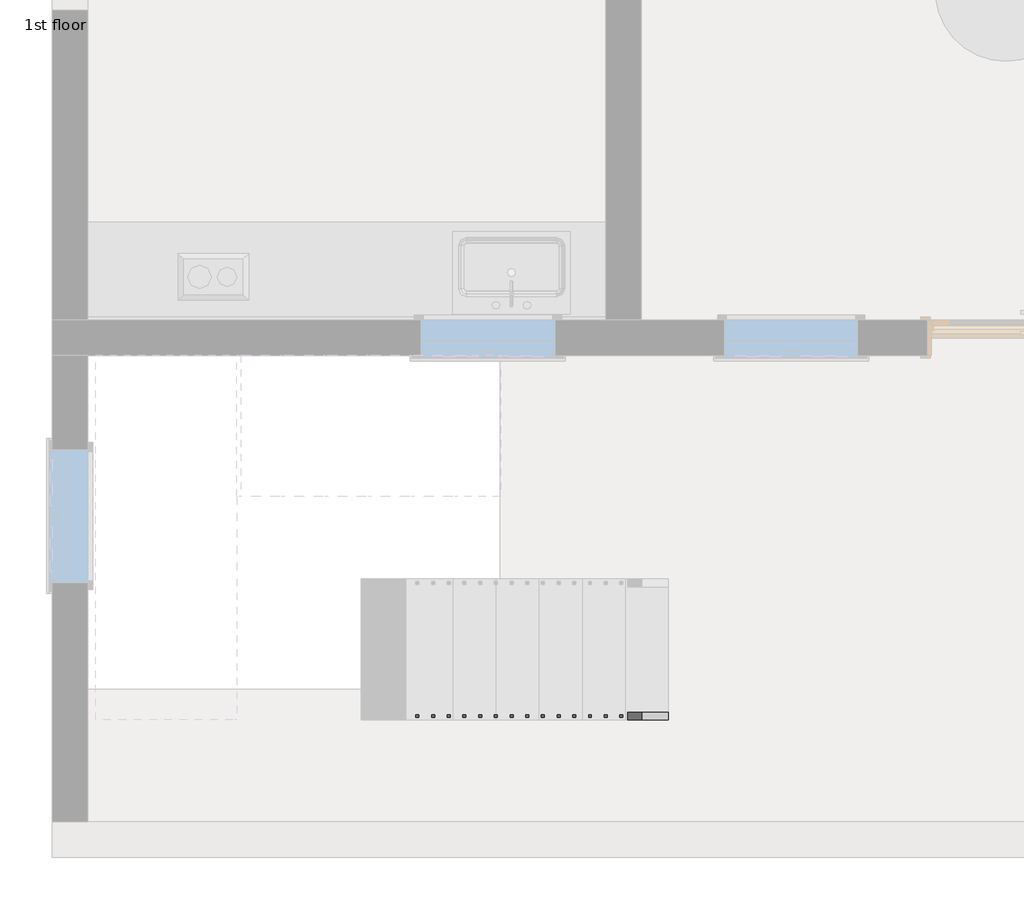
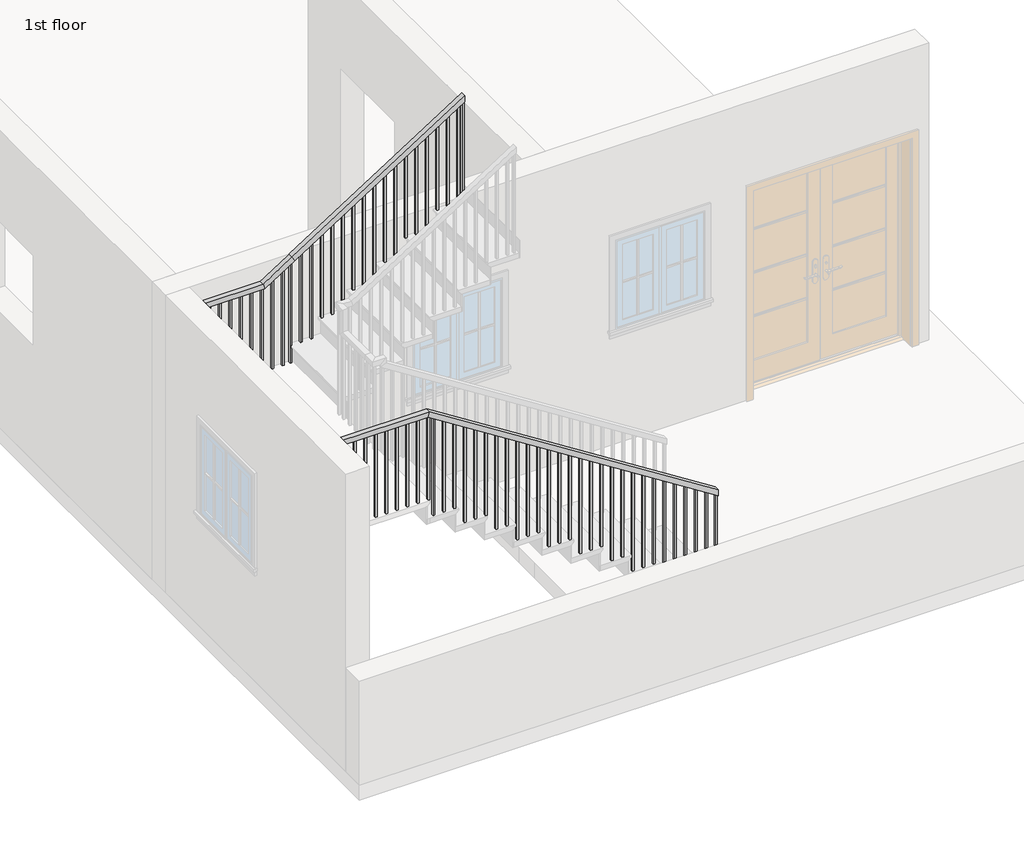
# One storey, part 2 of 3: 1 railing.
"""IFC4 building model written with IfcOpenShell, lengths in millimetres."""

from ifc_helpers import new_model, si_unit, frame, origin, place, context, project, spatial, polyline, outline, extrude, faceted_brep, element, save

model = new_model("IFC4")

# Units and contexts
model_context = context("Model", 3, world=origin())
ifc_project = project(units=[si_unit("LENGTHUNIT", "METRE", prefix="MILLI")], contexts=[model_context])

# Site, building, storey
site = spatial("IfcSite", under=ifc_project)
building = spatial("IfcBuilding", under=site)
storey = spatial("IfcBuildingStorey", under=building, Name="1st floor", Elevation=3810.0)

# Railing
placement = place(None, origin())
element("IfcRailing", 1, ObjectType="Handrail - Rectangular", at=placement, inside=storey, context=model_context, shape_type="SolidModel", body=[
    faceted_brep([(23001.1136801, 4166.5752787, 4902.2), (23001.1136801, 4166.5752787, 4841.986276), (23001.1136801, 4217.3752787, 4841.986276), (23001.1136801, 4217.3752787, 4902.2), (20207.1136801, 4166.5752787, 6680.2), (20192.3206852, 4166.5752787, 6629.4), (20192.3206852, 4217.3752787, 6629.4), (20207.1136801, 4217.3752787, 6680.2), (19292.7136801, 4166.5752787, 6680.2), (19292.7136801, 4166.5752787, 6629.4), (19343.5136801, 4217.3752787, 6629.4), (19343.5136801, 4217.3752787, 6680.2), (19292.7136801, 6528.7752787, 6680.2), (19292.7136801, 6528.7752787, 6629.4), (19343.5136801, 6477.9752787, 6629.4), (19343.5136801, 6477.9752787, 6680.2), (19927.7136801, 6528.7752787, 6680.2), (19942.506675, 6528.7752787, 6629.4), (19942.506675, 6477.9752787, 6629.4), (19927.7136801, 6477.9752787, 6680.2), (20207.1136801, 6528.7752787, 6858.0), (20234.3869551, 6528.7752787, 6815.1419964), (20234.3869551, 6477.9752787, 6815.1419964), (20207.1136801, 6477.9752787, 6858.0), (21883.5136801, 6528.7752787, 7924.8), (21883.5136801, 6477.9752787, 7924.8), (21883.5136801, 6477.9752787, 7864.586276), (21883.5136801, 6528.7752787, 7864.586276)], [[[0, 1, 2, 3]], [[1, 0, 4, 5]], [[2, 1, 5, 6]], [[3, 2, 6, 7]], [[0, 3, 7, 4]], [[5, 4, 8, 9]], [[6, 5, 9, 10]], [[7, 6, 10, 11]], [[4, 7, 11, 8]], [[9, 8, 12, 13]], [[10, 9, 13, 14]], [[11, 10, 14, 15]], [[8, 11, 15, 12]], [[13, 12, 16, 17]], [[14, 13, 17, 18]], [[15, 14, 18, 19]], [[12, 15, 19, 16]], [[17, 16, 20, 21]], [[18, 17, 21, 22]], [[19, 18, 22, 23]], [[16, 19, 23, 20]], [[24, 25, 26, 27]], [[21, 20, 24, 27]], [[22, 21, 27, 26]], [[23, 22, 26, 25]], [[20, 23, 25, 24]]]),
    extrude(outline(polyline([(7826.1976396, 21823.1886801), (6832.6, 21823.1886801), (6832.6, 21842.2386801), (7838.3203669, 21842.2386801), (7826.1976396, 21823.1886801)])), frame((0.0, 6493.8502787, 0.0), z_axis=(0.0, 1.0, 0.0), x_axis=(0.0, 0.0, 1.0)), (0.0, 0.0, 1.0), 19.05),
    extrude(outline(polyline([(7761.5430941, 21721.5886801), (6832.6, 21721.5886801), (6832.6, 21740.6386801), (7773.6658214, 21740.6386801), (7761.5430941, 21721.5886801)])), frame((0.0, 6493.8502787, 0.0), z_axis=(0.0, 1.0, 0.0), x_axis=(0.0, 0.0, 1.0)), (0.0, 0.0, 1.0), 19.05),
    extrude(outline(polyline([(7696.8885487, 21619.9886801), (6832.6, 21619.9886801), (6832.6, 21639.0386801), (7709.011276, 21639.0386801), (7696.8885487, 21619.9886801)])), frame((0.0, 6493.8502787, 0.0), z_axis=(0.0, 1.0, 0.0), x_axis=(0.0, 0.0, 1.0)), (0.0, 0.0, 1.0), 19.05),
    extrude(outline(polyline([(7632.2340032, 21518.3886801), (6654.8, 21518.3886801), (6654.8, 21537.4386801), (7644.3567305, 21537.4386801), (7632.2340032, 21518.3886801)])), frame((0.0, 6493.8502787, 0.0), z_axis=(0.0, 1.0, 0.0), x_axis=(0.0, 0.0, 1.0)), (0.0, 0.0, 1.0), 19.05),
    extrude(outline(polyline([(7567.5794578, 21416.7886801), (6654.8, 21416.7886801), (6654.8, 21435.8386801), (7579.7021851, 21435.8386801), (7567.5794578, 21416.7886801)])), frame((0.0, 6493.8502787, 0.0), z_axis=(0.0, 1.0, 0.0), x_axis=(0.0, 0.0, 1.0)), (0.0, 0.0, 1.0), 19.05),
    extrude(outline(polyline([(7502.9249123, 21315.1886801), (6654.8, 21315.1886801), (6654.8, 21334.2386801), (7515.0476396, 21334.2386801), (7502.9249123, 21315.1886801)])), frame((0.0, 6493.8502787, 0.0), z_axis=(0.0, 1.0, 0.0), x_axis=(0.0, 0.0, 1.0)), (0.0, 0.0, 1.0), 19.05),
    extrude(outline(polyline([(7438.2703669, 21213.5886801), (6477.0, 21213.5886801), (6477.0, 21232.6386801), (7450.3930941, 21232.6386801), (7438.2703669, 21213.5886801)])), frame((0.0, 6493.8502787, 0.0), z_axis=(0.0, 1.0, 0.0), x_axis=(0.0, 0.0, 1.0)), (0.0, 0.0, 1.0), 19.05),
    extrude(outline(polyline([(7373.6158214, 21111.9886801), (6477.0, 21111.9886801), (6477.0, 21131.0386801), (7385.7385487, 21131.0386801), (7373.6158214, 21111.9886801)])), frame((0.0, 6493.8502787, 0.0), z_axis=(0.0, 1.0, 0.0), x_axis=(0.0, 0.0, 1.0)), (0.0, 0.0, 1.0), 19.05),
    extrude(outline(polyline([(7308.961276, 21010.3886801), (6299.2, 21010.3886801), (6299.2, 21029.4386801), (7321.0840032, 21029.4386801), (7308.961276, 21010.3886801)])), frame((0.0, 6493.8502787, 0.0), z_axis=(0.0, 1.0, 0.0), x_axis=(0.0, 0.0, 1.0)), (0.0, 0.0, 1.0), 19.05),
    extrude(outline(polyline([(7244.3067305, 20908.7886801), (6299.2, 20908.7886801), (6299.2, 20927.8386801), (7256.4294578, 20927.8386801), (7244.3067305, 20908.7886801)])), frame((0.0, 6493.8502787, 0.0), z_axis=(0.0, 1.0, 0.0), x_axis=(0.0, 0.0, 1.0)), (0.0, 0.0, 1.0), 19.05),
    extrude(outline(polyline([(7179.6521851, 20807.1886801), (6299.2, 20807.1886801), (6299.2, 20826.2386801), (7191.7749123, 20826.2386801), (7179.6521851, 20807.1886801)])), frame((0.0, 6493.8502787, 0.0), z_axis=(0.0, 1.0, 0.0), x_axis=(0.0, 0.0, 1.0)), (0.0, 0.0, 1.0), 19.05),
    extrude(outline(polyline([(7114.9976396, 20705.5886801), (6121.4, 20705.5886801), (6121.4, 20724.6386801), (7127.1203669, 20724.6386801), (7114.9976396, 20705.5886801)])), frame((0.0, 6493.8502787, 0.0), z_axis=(0.0, 1.0, 0.0), x_axis=(0.0, 0.0, 1.0)), (0.0, 0.0, 1.0), 19.05),
    extrude(outline(polyline([(7050.3430941, 20603.9886801), (6121.4, 20603.9886801), (6121.4, 20623.0386801), (7062.4658214, 20623.0386801), (7050.3430941, 20603.9886801)])), frame((0.0, 6493.8502787, 0.0), z_axis=(0.0, 1.0, 0.0), x_axis=(0.0, 0.0, 1.0)), (0.0, 0.0, 1.0), 19.05),
    extrude(outline(polyline([(6985.6885487, 20502.3886801), (6121.4, 20502.3886801), (6121.4, 20521.4386801), (6997.811276, 20521.4386801), (6985.6885487, 20502.3886801)])), frame((0.0, 6493.8502787, 0.0), z_axis=(0.0, 1.0, 0.0), x_axis=(0.0, 0.0, 1.0)), (0.0, 0.0, 1.0), 19.05),
    extrude(outline(polyline([(6921.0340032, 20400.7886801), (5943.6, 20400.7886801), (5943.6, 20419.8386801), (6933.1567305, 20419.8386801), (6921.0340032, 20400.7886801)])), frame((0.0, 6493.8502787, 0.0), z_axis=(0.0, 1.0, 0.0), x_axis=(0.0, 0.0, 1.0)), (0.0, 0.0, 1.0), 19.05),
    extrude(outline(polyline([(6856.3794578, 20299.1886801), (5943.6, 20299.1886801), (5943.6, 20318.2386801), (6868.5021851, 20318.2386801), (6856.3794578, 20299.1886801)])), frame((0.0, 6493.8502787, 0.0), z_axis=(0.0, 1.0, 0.0), x_axis=(0.0, 0.0, 1.0)), (0.0, 0.0, 1.0), 19.05),
    extrude(outline(polyline([(6743.2340032, 20121.3886801), (5765.8, 20121.3886801), (5765.8, 20140.4386801), (6755.3567305, 20140.4386801), (6743.2340032, 20121.3886801)])), frame((0.0, 6493.8502787, 0.0), z_axis=(0.0, 1.0, 0.0), x_axis=(0.0, 0.0, 1.0)), (0.0, 0.0, 1.0), 19.05),
    extrude(outline(polyline([(6678.5794578, 20019.7886801), (5765.8, 20019.7886801), (5765.8, 20038.8386801), (6690.7021851, 20038.8386801), (6678.5794578, 20019.7886801)])), frame((0.0, 6493.8502787, 0.0), z_axis=(0.0, 1.0, 0.0), x_axis=(0.0, 0.0, 1.0)), (0.0, 0.0, 1.0), 19.05),
    extrude(outline(polyline([(19918.1886801, 6512.9002787), (19937.2386801, 6512.9002787), (19937.2386801, 6493.8502787), (19918.1886801, 6493.8502787), (19918.1886801, 6512.9002787)])), frame((0.0, 0.0, 5765.8), z_axis=(0.0, 0.0, 1.0), x_axis=(1.0, 0.0, 0.0)), (0.0, 0.0, 1.0), 863.6),
    extrude(outline(polyline([(19816.5886801, 6512.9002787), (19835.6386801, 6512.9002787), (19835.6386801, 6493.8502787), (19816.5886801, 6493.8502787), (19816.5886801, 6512.9002787)])), frame((0.0, 0.0, 5765.8), z_axis=(0.0, 0.0, 1.0), x_axis=(1.0, 0.0, 0.0)), (0.0, 0.0, 1.0), 863.6),
    extrude(outline(polyline([(19714.9886801, 6512.9002787), (19734.0386801, 6512.9002787), (19734.0386801, 6493.8502787), (19714.9886801, 6493.8502787), (19714.9886801, 6512.9002787)])), frame((0.0, 0.0, 5765.8), z_axis=(0.0, 0.0, 1.0), x_axis=(1.0, 0.0, 0.0)), (0.0, 0.0, 1.0), 863.6),
    extrude(outline(polyline([(19613.3886801, 6512.9002787), (19632.4386801, 6512.9002787), (19632.4386801, 6493.8502787), (19613.3886801, 6493.8502787), (19613.3886801, 6512.9002787)])), frame((0.0, 0.0, 5765.8), z_axis=(0.0, 0.0, 1.0), x_axis=(1.0, 0.0, 0.0)), (0.0, 0.0, 1.0), 863.6),
    extrude(outline(polyline([(19511.7886801, 6512.9002787), (19530.8386801, 6512.9002787), (19530.8386801, 6493.8502787), (19511.7886801, 6493.8502787), (19511.7886801, 6512.9002787)])), frame((0.0, 0.0, 5765.8), z_axis=(0.0, 0.0, 1.0), x_axis=(1.0, 0.0, 0.0)), (0.0, 0.0, 1.0), 863.6),
    extrude(outline(polyline([(19410.1886801, 6512.9002787), (19429.2386801, 6512.9002787), (19429.2386801, 6493.8502787), (19410.1886801, 6493.8502787), (19410.1886801, 6512.9002787)])), frame((0.0, 0.0, 5765.8), z_axis=(0.0, 0.0, 1.0), x_axis=(1.0, 0.0, 0.0)), (0.0, 0.0, 1.0), 863.6),
    extrude(outline(polyline([(19308.5886801, 6417.6502787), (19308.5886801, 6436.7002787), (19327.6386801, 6436.7002787), (19327.6386801, 6417.6502787), (19308.5886801, 6417.6502787)])), frame((0.0, 0.0, 5765.8), z_axis=(0.0, 0.0, 1.0), x_axis=(1.0, 0.0, 0.0)), (0.0, 0.0, 1.0), 863.6),
    extrude(outline(polyline([(19308.5886801, 6316.0502787), (19308.5886801, 6335.1002787), (19327.6386801, 6335.1002787), (19327.6386801, 6316.0502787), (19308.5886801, 6316.0502787)])), frame((0.0, 0.0, 5765.8), z_axis=(0.0, 0.0, 1.0), x_axis=(1.0, 0.0, 0.0)), (0.0, 0.0, 1.0), 863.6),
    extrude(outline(polyline([(19308.5886801, 6214.4502787), (19308.5886801, 6233.5002787), (19327.6386801, 6233.5002787), (19327.6386801, 6214.4502787), (19308.5886801, 6214.4502787)])), frame((0.0, 0.0, 5765.8), z_axis=(0.0, 0.0, 1.0), x_axis=(1.0, 0.0, 0.0)), (0.0, 0.0, 1.0), 863.6),
    extrude(outline(polyline([(19308.5886801, 6112.8502787), (19308.5886801, 6131.9002787), (19327.6386801, 6131.9002787), (19327.6386801, 6112.8502787), (19308.5886801, 6112.8502787)])), frame((0.0, 0.0, 5765.8), z_axis=(0.0, 0.0, 1.0), x_axis=(1.0, 0.0, 0.0)), (0.0, 0.0, 1.0), 863.6),
    extrude(outline(polyline([(19308.5886801, 6011.2502787), (19308.5886801, 6030.3002787), (19327.6386801, 6030.3002787), (19327.6386801, 6011.2502787), (19308.5886801, 6011.2502787)])), frame((0.0, 0.0, 5765.8), z_axis=(0.0, 0.0, 1.0), x_axis=(1.0, 0.0, 0.0)), (0.0, 0.0, 1.0), 863.6),
    extrude(outline(polyline([(19308.5886801, 5909.6502787), (19308.5886801, 5928.7002787), (19327.6386801, 5928.7002787), (19327.6386801, 5909.6502787), (19308.5886801, 5909.6502787)])), frame((0.0, 0.0, 5765.8), z_axis=(0.0, 0.0, 1.0), x_axis=(1.0, 0.0, 0.0)), (0.0, 0.0, 1.0), 863.6),
    extrude(outline(polyline([(19308.5886801, 5808.0502787), (19308.5886801, 5827.1002787), (19327.6386801, 5827.1002787), (19327.6386801, 5808.0502787), (19308.5886801, 5808.0502787)])), frame((0.0, 0.0, 5765.8), z_axis=(0.0, 0.0, 1.0), x_axis=(1.0, 0.0, 0.0)), (0.0, 0.0, 1.0), 863.6),
    extrude(outline(polyline([(19308.5886801, 5706.4502787), (19308.5886801, 5725.5002787), (19327.6386801, 5725.5002787), (19327.6386801, 5706.4502787), (19308.5886801, 5706.4502787)])), frame((0.0, 0.0, 5765.8), z_axis=(0.0, 0.0, 1.0), x_axis=(1.0, 0.0, 0.0)), (0.0, 0.0, 1.0), 863.6),
    extrude(outline(polyline([(19308.5886801, 5604.8502787), (19308.5886801, 5623.9002787), (19327.6386801, 5623.9002787), (19327.6386801, 5604.8502787), (19308.5886801, 5604.8502787)])), frame((0.0, 0.0, 5765.8), z_axis=(0.0, 0.0, 1.0), x_axis=(1.0, 0.0, 0.0)), (0.0, 0.0, 1.0), 863.6),
    extrude(outline(polyline([(19308.5886801, 5503.2502787), (19308.5886801, 5522.3002787), (19327.6386801, 5522.3002787), (19327.6386801, 5503.2502787), (19308.5886801, 5503.2502787)])), frame((0.0, 0.0, 5765.8), z_axis=(0.0, 0.0, 1.0), x_axis=(1.0, 0.0, 0.0)), (0.0, 0.0, 1.0), 863.6),
    extrude(outline(polyline([(19308.5886801, 5401.6502787), (19308.5886801, 5420.7002787), (19327.6386801, 5420.7002787), (19327.6386801, 5401.6502787), (19308.5886801, 5401.6502787)])), frame((0.0, 0.0, 5765.8), z_axis=(0.0, 0.0, 1.0), x_axis=(1.0, 0.0, 0.0)), (0.0, 0.0, 1.0), 863.6),
    extrude(outline(polyline([(19308.5886801, 5300.0502787), (19308.5886801, 5319.1002787), (19327.6386801, 5319.1002787), (19327.6386801, 5300.0502787), (19308.5886801, 5300.0502787)])), frame((0.0, 0.0, 5765.8), z_axis=(0.0, 0.0, 1.0), x_axis=(1.0, 0.0, 0.0)), (0.0, 0.0, 1.0), 863.6),
    extrude(outline(polyline([(19308.5886801, 5198.4502787), (19308.5886801, 5217.5002787), (19327.6386801, 5217.5002787), (19327.6386801, 5198.4502787), (19308.5886801, 5198.4502787)])), frame((0.0, 0.0, 5765.8), z_axis=(0.0, 0.0, 1.0), x_axis=(1.0, 0.0, 0.0)), (0.0, 0.0, 1.0), 863.6),
    extrude(outline(polyline([(19308.5886801, 5096.8502787), (19308.5886801, 5115.9002787), (19327.6386801, 5115.9002787), (19327.6386801, 5096.8502787), (19308.5886801, 5096.8502787)])), frame((0.0, 0.0, 5765.8), z_axis=(0.0, 0.0, 1.0), x_axis=(1.0, 0.0, 0.0)), (0.0, 0.0, 1.0), 863.6),
    extrude(outline(polyline([(19308.5886801, 4995.2502787), (19308.5886801, 5014.3002787), (19327.6386801, 5014.3002787), (19327.6386801, 4995.2502787), (19308.5886801, 4995.2502787)])), frame((0.0, 0.0, 5765.8), z_axis=(0.0, 0.0, 1.0), x_axis=(1.0, 0.0, 0.0)), (0.0, 0.0, 1.0), 863.6),
    extrude(outline(polyline([(19308.5886801, 4893.6502787), (19308.5886801, 4912.7002787), (19327.6386801, 4912.7002787), (19327.6386801, 4893.6502787), (19308.5886801, 4893.6502787)])), frame((0.0, 0.0, 5765.8), z_axis=(0.0, 0.0, 1.0), x_axis=(1.0, 0.0, 0.0)), (0.0, 0.0, 1.0), 863.6),
    extrude(outline(polyline([(19308.5886801, 4792.0502787), (19308.5886801, 4811.1002787), (19327.6386801, 4811.1002787), (19327.6386801, 4792.0502787), (19308.5886801, 4792.0502787)])), frame((0.0, 0.0, 5765.8), z_axis=(0.0, 0.0, 1.0), x_axis=(1.0, 0.0, 0.0)), (0.0, 0.0, 1.0), 863.6),
    extrude(outline(polyline([(19308.5886801, 4690.4502787), (19308.5886801, 4709.5002787), (19327.6386801, 4709.5002787), (19327.6386801, 4690.4502787), (19308.5886801, 4690.4502787)])), frame((0.0, 0.0, 5765.8), z_axis=(0.0, 0.0, 1.0), x_axis=(1.0, 0.0, 0.0)), (0.0, 0.0, 1.0), 863.6),
    extrude(outline(polyline([(19308.5886801, 4588.8502787), (19308.5886801, 4607.9002787), (19327.6386801, 4607.9002787), (19327.6386801, 4588.8502787), (19308.5886801, 4588.8502787)])), frame((0.0, 0.0, 5765.8), z_axis=(0.0, 0.0, 1.0), x_axis=(1.0, 0.0, 0.0)), (0.0, 0.0, 1.0), 863.6),
    extrude(outline(polyline([(19308.5886801, 4487.2502787), (19308.5886801, 4506.3002787), (19327.6386801, 4506.3002787), (19327.6386801, 4487.2502787), (19308.5886801, 4487.2502787)])), frame((0.0, 0.0, 5765.8), z_axis=(0.0, 0.0, 1.0), x_axis=(1.0, 0.0, 0.0)), (0.0, 0.0, 1.0), 863.6),
    extrude(outline(polyline([(19308.5886801, 4385.6502787), (19308.5886801, 4404.7002787), (19327.6386801, 4404.7002787), (19327.6386801, 4385.6502787), (19308.5886801, 4385.6502787)])), frame((0.0, 0.0, 5765.8), z_axis=(0.0, 0.0, 1.0), x_axis=(1.0, 0.0, 0.0)), (0.0, 0.0, 1.0), 863.6),
    extrude(outline(polyline([(19308.5886801, 4284.0502787), (19308.5886801, 4303.1002787), (19327.6386801, 4303.1002787), (19327.6386801, 4284.0502787), (19308.5886801, 4284.0502787)])), frame((0.0, 0.0, 5765.8), z_axis=(0.0, 0.0, 1.0), x_axis=(1.0, 0.0, 0.0)), (0.0, 0.0, 1.0), 863.6),
    extrude(outline(polyline([(19403.8386801, 4182.4502787), (19384.7886801, 4182.4502787), (19384.7886801, 4201.5002787), (19403.8386801, 4201.5002787), (19403.8386801, 4182.4502787)])), frame((0.0, 0.0, 5765.8), z_axis=(0.0, 0.0, 1.0), x_axis=(1.0, 0.0, 0.0)), (0.0, 0.0, 1.0), 863.6),
    extrude(outline(polyline([(19505.4386801, 4182.4502787), (19486.3886801, 4182.4502787), (19486.3886801, 4201.5002787), (19505.4386801, 4201.5002787), (19505.4386801, 4182.4502787)])), frame((0.0, 0.0, 5765.8), z_axis=(0.0, 0.0, 1.0), x_axis=(1.0, 0.0, 0.0)), (0.0, 0.0, 1.0), 863.6),
    extrude(outline(polyline([(19607.0386801, 4182.4502787), (19587.9886801, 4182.4502787), (19587.9886801, 4201.5002787), (19607.0386801, 4201.5002787), (19607.0386801, 4182.4502787)])), frame((0.0, 0.0, 5765.8), z_axis=(0.0, 0.0, 1.0), x_axis=(1.0, 0.0, 0.0)), (0.0, 0.0, 1.0), 863.6),
    extrude(outline(polyline([(19708.6386801, 4182.4502787), (19689.5886801, 4182.4502787), (19689.5886801, 4201.5002787), (19708.6386801, 4201.5002787), (19708.6386801, 4182.4502787)])), frame((0.0, 0.0, 5765.8), z_axis=(0.0, 0.0, 1.0), x_axis=(1.0, 0.0, 0.0)), (0.0, 0.0, 1.0), 863.6),
    extrude(outline(polyline([(19810.2386801, 4182.4502787), (19791.1886801, 4182.4502787), (19791.1886801, 4201.5002787), (19810.2386801, 4201.5002787), (19810.2386801, 4182.4502787)])), frame((0.0, 0.0, 5765.8), z_axis=(0.0, 0.0, 1.0), x_axis=(1.0, 0.0, 0.0)), (0.0, 0.0, 1.0), 863.6),
    extrude(outline(polyline([(19911.8386801, 4182.4502787), (19892.7886801, 4182.4502787), (19892.7886801, 4201.5002787), (19911.8386801, 4201.5002787), (19911.8386801, 4182.4502787)])), frame((0.0, 0.0, 5765.8), z_axis=(0.0, 0.0, 1.0), x_axis=(1.0, 0.0, 0.0)), (0.0, 0.0, 1.0), 863.6),
    extrude(outline(polyline([(20013.4386801, 4182.4502787), (19994.3886801, 4182.4502787), (19994.3886801, 4201.5002787), (20013.4386801, 4201.5002787), (20013.4386801, 4182.4502787)])), frame((0.0, 0.0, 5765.8), z_axis=(0.0, 0.0, 1.0), x_axis=(1.0, 0.0, 0.0)), (0.0, 0.0, 1.0), 863.6),
    extrude(outline(polyline([(20115.0386801, 4182.4502787), (20095.9886801, 4182.4502787), (20095.9886801, 4201.5002787), (20115.0386801, 4201.5002787), (20115.0386801, 4182.4502787)])), frame((0.0, 0.0, 5765.8), z_axis=(0.0, 0.0, 1.0), x_axis=(1.0, 0.0, 0.0)), (0.0, 0.0, 1.0), 863.6),
    extrude(outline(polyline([(6593.7203669, 20248.3886801), (5588.0, 20248.3886801), (5588.0, 20267.4386801), (6581.5976396, 20267.4386801), (6593.7203669, 20248.3886801)])), frame((0.0, 4182.4502787, 0.0), z_axis=(0.0, 1.0, 0.0), x_axis=(0.0, 0.0, 1.0)), (0.0, 0.0, 1.0), 19.05),
    extrude(outline(polyline([(6529.0658214, 20349.9886801), (5588.0, 20349.9886801), (5588.0, 20369.0386801), (6516.9430941, 20369.0386801), (6529.0658214, 20349.9886801)])), frame((0.0, 4182.4502787, 0.0), z_axis=(0.0, 1.0, 0.0), x_axis=(0.0, 0.0, 1.0)), (0.0, 0.0, 1.0), 19.05),
    extrude(outline(polyline([(6464.411276, 20451.5886801), (5588.0, 20451.5886801), (5588.0, 20470.6386801), (6452.2885487, 20470.6386801), (6464.411276, 20451.5886801)])), frame((0.0, 4182.4502787, 0.0), z_axis=(0.0, 1.0, 0.0), x_axis=(0.0, 0.0, 1.0)), (0.0, 0.0, 1.0), 19.05),
    extrude(outline(polyline([(6399.7567305, 20553.1886801), (5410.2, 20553.1886801), (5410.2, 20572.2386801), (6387.6340032, 20572.2386801), (6399.7567305, 20553.1886801)])), frame((0.0, 4182.4502787, 0.0), z_axis=(0.0, 1.0, 0.0), x_axis=(0.0, 0.0, 1.0)), (0.0, 0.0, 1.0), 19.05),
    extrude(outline(polyline([(6335.1021851, 20654.7886801), (5410.2, 20654.7886801), (5410.2, 20673.8386801), (6322.9794578, 20673.8386801), (6335.1021851, 20654.7886801)])), frame((0.0, 4182.4502787, 0.0), z_axis=(0.0, 1.0, 0.0), x_axis=(0.0, 0.0, 1.0)), (0.0, 0.0, 1.0), 19.05),
    extrude(outline(polyline([(6270.4476396, 20756.3886801), (5410.2, 20756.3886801), (5410.2, 20775.4386801), (6258.3249123, 20775.4386801), (6270.4476396, 20756.3886801)])), frame((0.0, 4182.4502787, 0.0), z_axis=(0.0, 1.0, 0.0), x_axis=(0.0, 0.0, 1.0)), (0.0, 0.0, 1.0), 19.05),
    extrude(outline(polyline([(6205.7930941, 20857.9886801), (5232.4, 20857.9886801), (5232.4, 20877.0386801), (6193.6703669, 20877.0386801), (6205.7930941, 20857.9886801)])), frame((0.0, 4182.4502787, 0.0), z_axis=(0.0, 1.0, 0.0), x_axis=(0.0, 0.0, 1.0)), (0.0, 0.0, 1.0), 19.05),
    extrude(outline(polyline([(6141.1385487, 20959.5886801), (5232.4, 20959.5886801), (5232.4, 20978.6386801), (6129.0158214, 20978.6386801), (6141.1385487, 20959.5886801)])), frame((0.0, 4182.4502787, 0.0), z_axis=(0.0, 1.0, 0.0), x_axis=(0.0, 0.0, 1.0)), (0.0, 0.0, 1.0), 19.05),
    extrude(outline(polyline([(6076.4840032, 21061.1886801), (5054.6, 21061.1886801), (5054.6, 21080.2386801), (6064.361276, 21080.2386801), (6076.4840032, 21061.1886801)])), frame((0.0, 4182.4502787, 0.0), z_axis=(0.0, 1.0, 0.0), x_axis=(0.0, 0.0, 1.0)), (0.0, 0.0, 1.0), 19.05),
    extrude(outline(polyline([(6011.8294578, 21162.7886801), (5054.6, 21162.7886801), (5054.6, 21181.8386801), (5999.7067305, 21181.8386801), (6011.8294578, 21162.7886801)])), frame((0.0, 4182.4502787, 0.0), z_axis=(0.0, 1.0, 0.0), x_axis=(0.0, 0.0, 1.0)), (0.0, 0.0, 1.0), 19.05),
    extrude(outline(polyline([(5947.1749123, 21264.3886801), (5054.6, 21264.3886801), (5054.6, 21283.4386801), (5935.0521851, 21283.4386801), (5947.1749123, 21264.3886801)])), frame((0.0, 4182.4502787, 0.0), z_axis=(0.0, 1.0, 0.0), x_axis=(0.0, 0.0, 1.0)), (0.0, 0.0, 1.0), 19.05),
    extrude(outline(polyline([(5882.5203669, 21365.9886801), (4876.8, 21365.9886801), (4876.8, 21385.0386801), (5870.3976396, 21385.0386801), (5882.5203669, 21365.9886801)])), frame((0.0, 4182.4502787, 0.0), z_axis=(0.0, 1.0, 0.0), x_axis=(0.0, 0.0, 1.0)), (0.0, 0.0, 1.0), 19.05),
    extrude(outline(polyline([(5817.8658214, 21467.5886801), (4876.8, 21467.5886801), (4876.8, 21486.6386801), (5805.7430941, 21486.6386801), (5817.8658214, 21467.5886801)])), frame((0.0, 4182.4502787, 0.0), z_axis=(0.0, 1.0, 0.0), x_axis=(0.0, 0.0, 1.0)), (0.0, 0.0, 1.0), 19.05),
    extrude(outline(polyline([(5753.211276, 21569.1886801), (4876.8, 21569.1886801), (4876.8, 21588.2386801), (5741.0885487, 21588.2386801), (5753.211276, 21569.1886801)])), frame((0.0, 4182.4502787, 0.0), z_axis=(0.0, 1.0, 0.0), x_axis=(0.0, 0.0, 1.0)), (0.0, 0.0, 1.0), 19.05),
    extrude(outline(polyline([(5688.5567305, 21670.7886801), (4699.0, 21670.7886801), (4699.0, 21689.8386801), (5676.4340032, 21689.8386801), (5688.5567305, 21670.7886801)])), frame((0.0, 4182.4502787, 0.0), z_axis=(0.0, 1.0, 0.0), x_axis=(0.0, 0.0, 1.0)), (0.0, 0.0, 1.0), 19.05),
    extrude(outline(polyline([(5623.9021851, 21772.3886801), (4699.0, 21772.3886801), (4699.0, 21791.4386801), (5611.7794578, 21791.4386801), (5623.9021851, 21772.3886801)])), frame((0.0, 4182.4502787, 0.0), z_axis=(0.0, 1.0, 0.0), x_axis=(0.0, 0.0, 1.0)), (0.0, 0.0, 1.0), 19.05),
    extrude(outline(polyline([(5559.2476396, 21873.9886801), (4699.0, 21873.9886801), (4699.0, 21893.0386801), (5547.1249123, 21893.0386801), (5559.2476396, 21873.9886801)])), frame((0.0, 4182.4502787, 0.0), z_axis=(0.0, 1.0, 0.0), x_axis=(0.0, 0.0, 1.0)), (0.0, 0.0, 1.0), 19.05),
    extrude(outline(polyline([(5494.5930941, 21975.5886801), (4521.2, 21975.5886801), (4521.2, 21994.6386801), (5482.4703669, 21994.6386801), (5494.5930941, 21975.5886801)])), frame((0.0, 4182.4502787, 0.0), z_axis=(0.0, 1.0, 0.0), x_axis=(0.0, 0.0, 1.0)), (0.0, 0.0, 1.0), 19.05),
    extrude(outline(polyline([(5429.9385487, 22077.1886801), (4521.2, 22077.1886801), (4521.2, 22096.2386801), (5417.8158214, 22096.2386801), (5429.9385487, 22077.1886801)])), frame((0.0, 4182.4502787, 0.0), z_axis=(0.0, 1.0, 0.0), x_axis=(0.0, 0.0, 1.0)), (0.0, 0.0, 1.0), 19.05),
    extrude(outline(polyline([(5365.2840032, 22178.7886801), (4343.4, 22178.7886801), (4343.4, 22197.8386801), (5353.161276, 22197.8386801), (5365.2840032, 22178.7886801)])), frame((0.0, 4182.4502787, 0.0), z_axis=(0.0, 1.0, 0.0), x_axis=(0.0, 0.0, 1.0)), (0.0, 0.0, 1.0), 19.05),
    extrude(outline(polyline([(5300.6294578, 22280.3886801), (4343.4, 22280.3886801), (4343.4, 22299.4386801), (5288.5067305, 22299.4386801), (5300.6294578, 22280.3886801)])), frame((0.0, 4182.4502787, 0.0), z_axis=(0.0, 1.0, 0.0), x_axis=(0.0, 0.0, 1.0)), (0.0, 0.0, 1.0), 19.05),
    extrude(outline(polyline([(5235.9749123, 22381.9886801), (4343.4, 22381.9886801), (4343.4, 22401.0386801), (5223.8521851, 22401.0386801), (5235.9749123, 22381.9886801)])), frame((0.0, 4182.4502787, 0.0), z_axis=(0.0, 1.0, 0.0), x_axis=(0.0, 0.0, 1.0)), (0.0, 0.0, 1.0), 19.05),
    extrude(outline(polyline([(5171.3203669, 22483.5886801), (4165.6, 22483.5886801), (4165.6, 22502.6386801), (5159.1976396, 22502.6386801), (5171.3203669, 22483.5886801)])), frame((0.0, 4182.4502787, 0.0), z_axis=(0.0, 1.0, 0.0), x_axis=(0.0, 0.0, 1.0)), (0.0, 0.0, 1.0), 19.05),
    extrude(outline(polyline([(5106.6658214, 22585.1886801), (4165.6, 22585.1886801), (4165.6, 22604.2386801), (5094.5430941, 22604.2386801), (5106.6658214, 22585.1886801)])), frame((0.0, 4182.4502787, 0.0), z_axis=(0.0, 1.0, 0.0), x_axis=(0.0, 0.0, 1.0)), (0.0, 0.0, 1.0), 19.05),
    extrude(outline(polyline([(5042.011276, 22686.7886801), (4165.6, 22686.7886801), (4165.6, 22705.8386801), (5029.8885487, 22705.8386801), (5042.011276, 22686.7886801)])), frame((0.0, 4182.4502787, 0.0), z_axis=(0.0, 1.0, 0.0), x_axis=(0.0, 0.0, 1.0)), (0.0, 0.0, 1.0), 19.05),
    extrude(outline(polyline([(4977.3567305, 22788.3886801), (3987.8, 22788.3886801), (3987.8, 22807.4386801), (4965.2340032, 22807.4386801), (4977.3567305, 22788.3886801)])), frame((0.0, 4182.4502787, 0.0), z_axis=(0.0, 1.0, 0.0), x_axis=(0.0, 0.0, 1.0)), (0.0, 0.0, 1.0), 19.05),
    extrude(outline(polyline([(4912.7021851, 22889.9886801), (3987.8, 22889.9886801), (3987.8, 22909.0386801), (4900.5794578, 22909.0386801), (4912.7021851, 22889.9886801)])), frame((0.0, 4182.4502787, 0.0), z_axis=(0.0, 1.0, 0.0), x_axis=(0.0, 0.0, 1.0)), (0.0, 0.0, 1.0), 19.05),
    extrude(outline(polyline([(6791.7249123, 20197.5886801), (5765.8, 20197.5886801), (5765.8, 20216.6386801), (6803.8476396, 20216.6386801), (6791.7249123, 20197.5886801)])), frame((0.0, 6493.8502787, 0.0), z_axis=(0.0, 1.0, 0.0), x_axis=(0.0, 0.0, 1.0)), (0.0, 0.0, 1.0), 19.05),
    extrude(outline(polyline([(19308.5886801, 6493.8502787), (19308.5886801, 6512.9002787), (19327.6386801, 6512.9002787), (19327.6386801, 6493.8502787), (19308.5886801, 6493.8502787)])), frame((0.0, 0.0, 5765.8), z_axis=(0.0, 0.0, 1.0), x_axis=(1.0, 0.0, 0.0)), (0.0, 0.0, 1.0), 863.6),
    extrude(outline(polyline([(19327.6386801, 4182.4502787), (19308.5886801, 4182.4502787), (19308.5886801, 4201.5002787), (19327.6386801, 4201.5002787), (19327.6386801, 4182.4502787)])), frame((0.0, 0.0, 5765.8), z_axis=(0.0, 0.0, 1.0), x_axis=(1.0, 0.0, 0.0)), (0.0, 0.0, 1.0), 863.6),
    extrude(outline(polyline([(6626.0476396, 20197.5886801), (5765.8, 20197.5886801), (5765.8, 20216.6386801), (6613.9249123, 20216.6386801), (6626.0476396, 20197.5886801)])), frame((0.0, 4182.4502787, 0.0), z_axis=(0.0, 1.0, 0.0), x_axis=(0.0, 0.0, 1.0)), (0.0, 0.0, 1.0), 19.05),
    extrude(outline(polyline([(7852.4635487, 21864.4636801), (6832.6, 21864.4636801), (6832.6, 21883.5136801), (7864.586276, 21883.5136801), (7852.4635487, 21864.4636801)])), frame((0.0, 6493.8502787, 0.0), z_axis=(0.0, 1.0, 0.0), x_axis=(0.0, 0.0, 1.0)), (0.0, 0.0, 1.0), 19.05),
    extrude(outline(polyline([(4854.1090032, 22982.0636801), (3987.8, 22982.0636801), (3987.8, 23001.1136801), (4841.986276, 23001.1136801), (4854.1090032, 22982.0636801)])), frame((0.0, 4182.4502787, 0.0), z_axis=(0.0, 1.0, 0.0), x_axis=(0.0, 0.0, 1.0)), (0.0, 0.0, 1.0), 19.05),
])

save(model, "model.ifc")

# Revit data of these elements
# Type "Handrail - Rectangular"
#   Assembly Code = "C2010400"
#   built-in parameter 1008612 = 0.0416667 (stored number, unit not read)
#   built-in parameter 1008611 = 0.0416667 (stored number, unit not read)
#   built-in parameter 1008609 = 0.333333 (stored number, unit not read)
#   built-in parameter 1008604 = 0.166667 (stored number, unit not read)
#   built-in parameter 1008603 = 0.166667 (stored number, unit not read)
#   Railing Height = 3' - 0"
#   built-in parameter 1008630 = 2
#   built-in parameter 1008610 = 2
#   built-in parameter 1008618 = Baluster - Square : 3/4"
# Element 1 (IfcRailing, "Handrail - Rectangular")
#   Phase Created = New Construction
